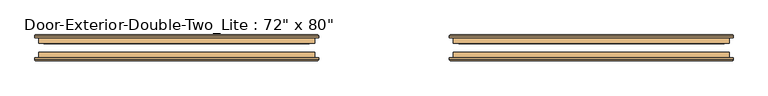
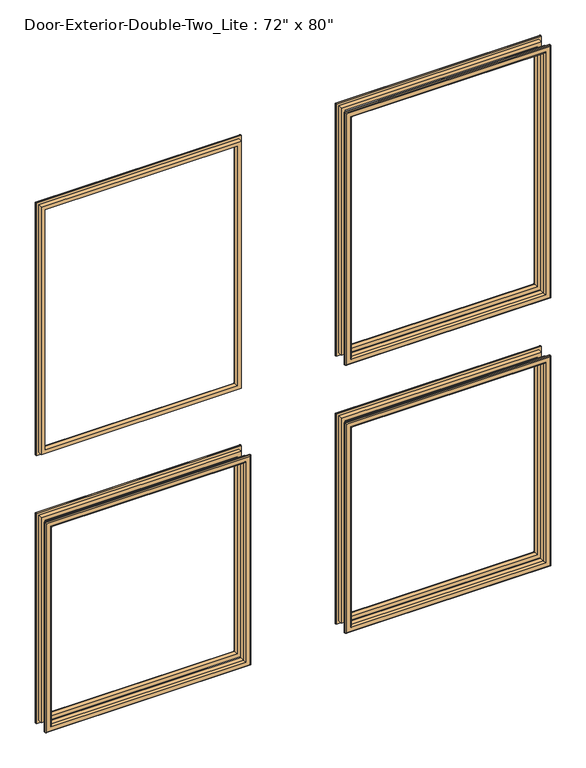
"""IFC4 building model written with IfcOpenShell, lengths in millimetres: door geometry."""

from ifc_helpers import new_model, si_unit, frame, origin, place, context, project, spatial, ellipse_curve, source, transform, mapped, element, save
from ifc_brep_helpers import plane_surface, cylinder_surface, advanced_brep


def door_cb6735bc(model_context):
    return source(origin(), model_context, "Body", "AdvancedBrep", [
        advanced_brep(
        [(-762.0, 69.85, 914.4), (-762.0, 82.55, 914.4), (-762.0, 82.55, 254.0), (-762.0, 69.85, 254.0), (-750.0, 83.55, 902.4), (-750.0, 69.85, 902.4), (-750.0, 69.85, 266.0), (-750.0, 83.55, 266.0), (-755.0, 88.55, 907.4), (-755.0, 88.55, 261.0), (-770.0, 86.55, 922.4), (-768.0, 88.55, 920.4), (-768.0, 88.55, 248.0), (-770.0, 86.55, 246.0), (-770.0, 82.55, 922.4), (-770.0, 82.55, 246.0), (-152.4, 82.55, 254.0), (-152.4, 69.85, 254.0), (-164.4, 69.85, 266.0), (-164.4, 83.55, 266.0), (-159.4, 88.55, 261.0), (-146.4, 88.55, 248.0), (-144.4, 86.55, 246.0), (-144.4, 82.55, 246.0), (-152.4, 82.55, 914.4), (-152.4, 69.85, 914.4), (-164.4, 69.85, 902.4), (-164.4, 83.55, 902.4), (-159.4, 88.55, 907.4), (-146.4, 88.55, 920.4), (-144.4, 86.55, 922.4), (-144.4, 82.55, 922.4)],
        [
            (0, 1),
            (1, 2),
            (2, 3),
            (3, 0),
            (4, 5),
            (5, 6),
            (6, 7),
            (7, 4),
            (8, 4, ellipse_curve(frame((-755.0, 83.55, 907.4), z_axis=(-0.7071067811865475, 0.0, -0.7071067811865475), x_axis=(-0.7071067811865474, 0.0, 0.7071067811865476)), 7.0710678, 5.0)),
            (7, 9, ellipse_curve(frame((-755.0, 83.55, 261.0), z_axis=(-0.7071067811865475, 0.0, 0.7071067811865475), x_axis=(0.7071067811865474, 0.0, 0.7071067811865476)), 7.0710678, 5.0)),
            (9, 8),
            (10, 11, ellipse_curve(frame((-768.0, 86.55, 920.4), z_axis=(-0.7071067811865475, 0.0, -0.7071067811865475), x_axis=(-0.7071067811865474, 0.0, 0.7071067811865476)), 2.8284271, 2.0)),
            (11, 12),
            (12, 13, ellipse_curve(frame((-768.0, 86.55, 248.0), z_axis=(-0.7071067811865475, 0.0, 0.7071067811865475), x_axis=(0.7071067811865474, 0.0, 0.7071067811865476)), 2.8284271, 2.0)),
            (13, 10),
            (14, 10),
            (13, 15),
            (15, 14),
            (2, 16),
            (16, 17),
            (17, 3),
            (6, 18),
            (18, 19),
            (19, 7),
            (19, 20, ellipse_curve(frame((-159.4, 83.55, 261.0), z_axis=(-0.7071067811865475, 0.0, -0.7071067811865475), x_axis=(-0.7071067811865476, 0.0, 0.7071067811865474)), 7.0710678, 5.0)),
            (20, 9),
            (12, 21),
            (21, 22, ellipse_curve(frame((-146.4, 86.55, 248.0), z_axis=(-0.7071067811865475, 0.0, -0.7071067811865475), x_axis=(-0.7071067811865476, 0.0, 0.7071067811865474)), 2.8284271, 2.0)),
            (22, 13),
            (22, 23),
            (23, 15),
            (16, 24),
            (24, 25),
            (25, 17),
            (18, 26),
            (26, 27),
            (27, 19),
            (27, 28, ellipse_curve(frame((-159.4, 83.55, 907.4), z_axis=(0.7071067811865475, 0.0, -0.7071067811865475), x_axis=(-0.7071067811865474, 0.0, -0.7071067811865476)), 7.0710678, 5.0)),
            (28, 20),
            (21, 29),
            (29, 30, ellipse_curve(frame((-146.4, 86.55, 920.4), z_axis=(0.7071067811865475, 0.0, -0.7071067811865475), x_axis=(-0.7071067811865474, 0.0, -0.7071067811865476)), 2.8284271, 2.0)),
            (30, 22),
            (30, 31),
            (31, 23),
            (31, 14),
            (1, 24),
            (0, 25),
            (5, 26),
            (4, 27),
            (8, 28),
            (11, 29),
            (10, 30),
        ],
        [
            plane_surface(frame((-762.0, 82.55, 914.4), z_axis=(-1.0, 0.0, 0.0), x_axis=(0.0, 0.0, -1.0))),
            plane_surface(frame((-750.0, 69.85, 902.4), z_axis=(1.0, 0.0, 0.0), x_axis=(0.0, 0.0, -1.0))),
            cylinder_surface(frame((-755.0, 83.55, 914.4), z_axis=(0.0, 0.0, 1.0), x_axis=(-1.0, 0.0, 0.0)), 5.0),
            cylinder_surface(frame((-768.0, 86.55, 914.4), z_axis=(0.0, 0.0, 1.0), x_axis=(-1.0, 0.0, 0.0)), 2.0),
            plane_surface(frame((-770.0, 86.55, 922.4), z_axis=(-1.0, 0.0, 0.0), x_axis=(0.0, 0.0, -1.0))),
            plane_surface(frame((-762.0, 82.55, 254.0), z_axis=(0.0, 0.0, -1.0), x_axis=(1.0, 0.0, 0.0))),
            plane_surface(frame((-750.0, 69.85, 266.0), z_axis=(0.0, 0.0, 1.0), x_axis=(1.0, 0.0, 0.0))),
            cylinder_surface(frame((-762.0, 83.55, 261.0), z_axis=(-1.0, 0.0, 0.0), x_axis=(0.0, 0.0, -1.0)), 5.0),
            cylinder_surface(frame((-762.0, 86.55, 248.0), z_axis=(-1.0, 0.0, 0.0), x_axis=(0.0, 0.0, -1.0)), 2.0),
            plane_surface(frame((-770.0, 86.55, 246.0), z_axis=(0.0, 0.0, -1.0), x_axis=(1.0, 0.0, 0.0))),
            plane_surface(frame((-152.4, 82.55, 254.0), z_axis=(1.0, 0.0, 0.0), x_axis=(0.0, 0.0, 1.0))),
            plane_surface(frame((-164.4, 69.85, 266.0), z_axis=(-1.0, 0.0, 0.0), x_axis=(0.0, 0.0, 1.0))),
            cylinder_surface(frame((-159.4, 83.55, 254.0), z_axis=(0.0, 0.0, -1.0), x_axis=(1.0, 0.0, 0.0)), 5.0),
            cylinder_surface(frame((-146.4, 86.55, 254.0), z_axis=(0.0, 0.0, -1.0), x_axis=(1.0, 0.0, 0.0)), 2.0),
            plane_surface(frame((-144.4, 86.55, 246.0), z_axis=(1.0, 0.0, 0.0), x_axis=(0.0, 0.0, 1.0))),
            plane_surface(frame((-144.4, 82.55, 922.4), z_axis=(0.0, -1.0, 0.0), x_axis=(-1.0, 0.0, 0.0))),
            plane_surface(frame((-152.4, 82.55, 914.4), z_axis=(0.0, 0.0, 1.0), x_axis=(-1.0, 0.0, 0.0))),
            plane_surface(frame((-152.4, 69.85, 914.4), z_axis=(0.0, -1.0, 0.0), x_axis=(-1.0, 0.0, 0.0))),
            plane_surface(frame((-164.4, 69.85, 902.4), z_axis=(0.0, 0.0, -1.0), x_axis=(-1.0, 0.0, 0.0))),
            cylinder_surface(frame((-152.4, 83.55, 907.4), z_axis=(1.0, 0.0, 0.0), x_axis=(0.0, 0.0, 1.0)), 5.0),
            plane_surface(frame((-159.4, 88.55, 907.4), z_axis=(0.0, 1.0, 0.0), x_axis=(-1.0, 0.0, 0.0))),
            cylinder_surface(frame((-152.4, 86.55, 920.4), z_axis=(1.0, 0.0, 0.0), x_axis=(0.0, 0.0, 1.0)), 2.0),
            plane_surface(frame((-144.4, 86.55, 922.4), z_axis=(0.0, 0.0, 1.0), x_axis=(-1.0, 0.0, 0.0))),
        ],
        [
            (0, [[1, 2, 3, 4]]),
            (1, [[5, 6, 7, 8]]),
            (2, [[9, -8, 10, 11]]),
            (3, [[12, 13, 14, 15]]),
            (4, [[16, -15, 17, 18]]),
            (5, [[-3, 19, 20, 21]]),
            (6, [[-7, 22, 23, 24]]),
            (7, [[-10, -24, 25, 26]]),
            (8, [[-14, 27, 28, 29]]),
            (9, [[-17, -29, 30, 31]]),
            (10, [[-20, 32, 33, 34]]),
            (11, [[-23, 35, 36, 37]]),
            (12, [[-25, -37, 38, 39]]),
            (13, [[-28, 40, 41, 42]]),
            (14, [[-30, -42, 43, 44]]),
            (15, [[-31, -44, 45, -18], [46, -32, -19, -2]]),
            (16, [[-33, -46, -1, 47]]),
            (17, [[-21, -34, -47, -4], [48, -35, -22, -6]]),
            (18, [[-36, -48, -5, 49]]),
            (19, [[-38, -49, -9, 50]]),
            (20, [[51, -40, -27, -13], [-26, -39, -50, -11]]),
            (21, [[-41, -51, -12, 52]]),
            (22, [[-43, -52, -16, -45]]),
        ],
    ),
        advanced_brep(
        [(152.4, 69.85, 914.4), (152.4, 82.55, 914.4), (152.4, 82.55, 254.0), (152.4, 69.85, 254.0), (164.4, 83.55, 902.4), (164.4, 69.85, 902.4), (164.4, 69.85, 266.0), (164.4, 83.55, 266.0), (159.4, 88.55, 907.4), (159.4, 88.55, 261.0), (144.4, 86.55, 922.4), (146.4, 88.55, 920.4), (146.4, 88.55, 248.0), (144.4, 86.55, 246.0), (144.4, 82.55, 922.4), (144.4, 82.55, 246.0), (762.0, 82.55, 254.0), (762.0, 69.85, 254.0), (750.0, 69.85, 266.0), (750.0, 83.55, 266.0), (755.0, 88.55, 261.0), (768.0, 88.55, 248.0), (770.0, 86.55, 246.0), (770.0, 82.55, 246.0), (762.0, 82.55, 914.4), (762.0, 69.85, 914.4), (750.0, 69.85, 902.4), (750.0, 83.55, 902.4), (755.0, 88.55, 907.4), (768.0, 88.55, 920.4), (770.0, 86.55, 922.4), (770.0, 82.55, 922.4)],
        [
            (0, 1),
            (1, 2),
            (2, 3),
            (3, 0),
            (4, 5),
            (5, 6),
            (6, 7),
            (7, 4),
            (8, 4, ellipse_curve(frame((159.4, 83.55, 907.4), z_axis=(-0.7071067811865475, 0.0, -0.7071067811865475), x_axis=(-0.7071067811865474, 0.0, 0.7071067811865476)), 7.0710678, 5.0)),
            (7, 9, ellipse_curve(frame((159.4, 83.55, 261.0), z_axis=(-0.7071067811865475, 0.0, 0.7071067811865475), x_axis=(0.7071067811865474, 0.0, 0.7071067811865476)), 7.0710678, 5.0)),
            (9, 8),
            (10, 11, ellipse_curve(frame((146.4, 86.55, 920.4), z_axis=(-0.7071067811865475, 0.0, -0.7071067811865475), x_axis=(-0.7071067811865474, 0.0, 0.7071067811865476)), 2.8284271, 2.0)),
            (11, 12),
            (12, 13, ellipse_curve(frame((146.4, 86.55, 248.0), z_axis=(-0.7071067811865475, 0.0, 0.7071067811865475), x_axis=(0.7071067811865474, 0.0, 0.7071067811865476)), 2.8284271, 2.0)),
            (13, 10),
            (14, 10),
            (13, 15),
            (15, 14),
            (2, 16),
            (16, 17),
            (17, 3),
            (6, 18),
            (18, 19),
            (19, 7),
            (19, 20, ellipse_curve(frame((755.0, 83.55, 261.0), z_axis=(-0.7071067811865475, 0.0, -0.7071067811865475), x_axis=(-0.7071067811865476, 0.0, 0.7071067811865474)), 7.0710678, 5.0)),
            (20, 9),
            (12, 21),
            (21, 22, ellipse_curve(frame((768.0, 86.55, 248.0), z_axis=(-0.7071067811865475, 0.0, -0.7071067811865475), x_axis=(-0.7071067811865476, 0.0, 0.7071067811865474)), 2.8284271, 2.0)),
            (22, 13),
            (22, 23),
            (23, 15),
            (16, 24),
            (24, 25),
            (25, 17),
            (18, 26),
            (26, 27),
            (27, 19),
            (27, 28, ellipse_curve(frame((755.0, 83.55, 907.4), z_axis=(0.7071067811865475, 0.0, -0.7071067811865475), x_axis=(-0.7071067811865474, 0.0, -0.7071067811865476)), 7.0710678, 5.0)),
            (28, 20),
            (21, 29),
            (29, 30, ellipse_curve(frame((768.0, 86.55, 920.4), z_axis=(0.7071067811865475, 0.0, -0.7071067811865475), x_axis=(-0.7071067811865474, 0.0, -0.7071067811865476)), 2.8284271, 2.0)),
            (30, 22),
            (30, 31),
            (31, 23),
            (31, 14),
            (1, 24),
            (0, 25),
            (5, 26),
            (4, 27),
            (8, 28),
            (11, 29),
            (10, 30),
        ],
        [
            plane_surface(frame((152.4, 82.55, 914.4), z_axis=(-1.0, 0.0, 0.0), x_axis=(0.0, 0.0, -1.0))),
            plane_surface(frame((164.4, 69.85, 902.4), z_axis=(1.0, 0.0, 0.0), x_axis=(0.0, 0.0, -1.0))),
            cylinder_surface(frame((159.4, 83.55, 914.4), z_axis=(0.0, 0.0, 1.0), x_axis=(-1.0, 0.0, 0.0)), 5.0),
            cylinder_surface(frame((146.4, 86.55, 914.4), z_axis=(0.0, 0.0, 1.0), x_axis=(-1.0, 0.0, 0.0)), 2.0),
            plane_surface(frame((144.4, 86.55, 922.4), z_axis=(-1.0, 0.0, 0.0), x_axis=(0.0, 0.0, -1.0))),
            plane_surface(frame((152.4, 82.55, 254.0), z_axis=(0.0, 0.0, -1.0), x_axis=(1.0, 0.0, 0.0))),
            plane_surface(frame((164.4, 69.85, 266.0), z_axis=(0.0, 0.0, 1.0), x_axis=(1.0, 0.0, 0.0))),
            cylinder_surface(frame((152.4, 83.55, 261.0), z_axis=(-1.0, 0.0, 0.0), x_axis=(0.0, 0.0, -1.0)), 5.0),
            cylinder_surface(frame((152.4, 86.55, 248.0), z_axis=(-1.0, 0.0, 0.0), x_axis=(0.0, 0.0, -1.0)), 2.0),
            plane_surface(frame((144.4, 86.55, 246.0), z_axis=(0.0, 0.0, -1.0), x_axis=(1.0, 0.0, 0.0))),
            plane_surface(frame((762.0, 82.55, 254.0), z_axis=(1.0, 0.0, 0.0), x_axis=(0.0, 0.0, 1.0))),
            plane_surface(frame((750.0, 69.85, 266.0), z_axis=(-1.0, 0.0, 0.0), x_axis=(0.0, 0.0, 1.0))),
            cylinder_surface(frame((755.0, 83.55, 254.0), z_axis=(0.0, 0.0, -1.0), x_axis=(1.0, 0.0, 0.0)), 5.0),
            cylinder_surface(frame((768.0, 86.55, 254.0), z_axis=(0.0, 0.0, -1.0), x_axis=(1.0, 0.0, 0.0)), 2.0),
            plane_surface(frame((770.0, 86.55, 246.0), z_axis=(1.0, 0.0, 0.0), x_axis=(0.0, 0.0, 1.0))),
            plane_surface(frame((770.0, 82.55, 922.4), z_axis=(0.0, -1.0, 0.0), x_axis=(-1.0, 0.0, 0.0))),
            plane_surface(frame((762.0, 82.55, 914.4), z_axis=(0.0, 0.0, 1.0), x_axis=(-1.0, 0.0, 0.0))),
            plane_surface(frame((762.0, 69.85, 914.4), z_axis=(0.0, -1.0, 0.0), x_axis=(-1.0, 0.0, 0.0))),
            plane_surface(frame((750.0, 69.85, 902.4), z_axis=(0.0, 0.0, -1.0), x_axis=(-1.0, 0.0, 0.0))),
            cylinder_surface(frame((762.0, 83.55, 907.4), z_axis=(1.0, 0.0, 0.0), x_axis=(0.0, 0.0, 1.0)), 5.0),
            plane_surface(frame((755.0, 88.55, 907.4), z_axis=(0.0, 1.0, 0.0), x_axis=(-1.0, 0.0, 0.0))),
            cylinder_surface(frame((762.0, 86.55, 920.4), z_axis=(1.0, 0.0, 0.0), x_axis=(0.0, 0.0, 1.0)), 2.0),
            plane_surface(frame((770.0, 86.55, 922.4), z_axis=(0.0, 0.0, 1.0), x_axis=(-1.0, 0.0, 0.0))),
        ],
        [
            (0, [[1, 2, 3, 4]]),
            (1, [[5, 6, 7, 8]]),
            (2, [[9, -8, 10, 11]]),
            (3, [[12, 13, 14, 15]]),
            (4, [[16, -15, 17, 18]]),
            (5, [[-3, 19, 20, 21]]),
            (6, [[-7, 22, 23, 24]]),
            (7, [[-10, -24, 25, 26]]),
            (8, [[-14, 27, 28, 29]]),
            (9, [[-17, -29, 30, 31]]),
            (10, [[-20, 32, 33, 34]]),
            (11, [[-23, 35, 36, 37]]),
            (12, [[-25, -37, 38, 39]]),
            (13, [[-28, 40, 41, 42]]),
            (14, [[-30, -42, 43, 44]]),
            (15, [[-31, -44, 45, -18], [46, -32, -19, -2]]),
            (16, [[-33, -46, -1, 47]]),
            (17, [[-21, -34, -47, -4], [48, -35, -22, -6]]),
            (18, [[-36, -48, -5, 49]]),
            (19, [[-38, -49, -9, 50]]),
            (20, [[51, -40, -27, -13], [-26, -39, -50, -11]]),
            (21, [[-41, -51, -12, 52]]),
            (22, [[-43, -52, -16, -45]]),
        ],
    ),
        advanced_brep(
        [(152.4, 69.85, 1914.525), (152.4, 82.55, 1914.525), (152.4, 82.55, 1117.6), (152.4, 69.85, 1117.6), (164.4, 83.55, 1902.525), (164.4, 69.85, 1902.525), (164.4, 69.85, 1129.6), (164.4, 83.55, 1129.6), (159.4, 88.55, 1907.525), (159.4, 88.55, 1124.6), (144.4, 86.55, 1922.525), (146.4, 88.55, 1920.525), (146.4, 88.55, 1111.6), (144.4, 86.55, 1109.6), (144.4, 82.55, 1922.525), (144.4, 82.55, 1109.6), (762.0, 82.55, 1117.6), (762.0, 69.85, 1117.6), (750.0, 69.85, 1129.6), (750.0, 83.55, 1129.6), (755.0, 88.55, 1124.6), (768.0, 88.55, 1111.6), (770.0, 86.55, 1109.6), (770.0, 82.55, 1109.6), (762.0, 82.55, 1914.525), (762.0, 69.85, 1914.525), (750.0, 69.85, 1902.525), (750.0, 83.55, 1902.525), (755.0, 88.55, 1907.525), (768.0, 88.55, 1920.525), (770.0, 86.55, 1922.525), (770.0, 82.55, 1922.525)],
        [
            (0, 1),
            (1, 2),
            (2, 3),
            (3, 0),
            (4, 5),
            (5, 6),
            (6, 7),
            (7, 4),
            (8, 4, ellipse_curve(frame((159.4, 83.55, 1907.525), z_axis=(-0.7071067811865475, 0.0, -0.7071067811865475), x_axis=(-0.7071067811865474, 0.0, 0.7071067811865476)), 7.0710678, 5.0)),
            (7, 9, ellipse_curve(frame((159.4, 83.55, 1124.6), z_axis=(-0.7071067811865475, 0.0, 0.7071067811865475), x_axis=(0.7071067811865474, 0.0, 0.7071067811865476)), 7.0710678, 5.0)),
            (9, 8),
            (10, 11, ellipse_curve(frame((146.4, 86.55, 1920.525), z_axis=(-0.7071067811865475, 0.0, -0.7071067811865475), x_axis=(-0.7071067811865474, 0.0, 0.7071067811865476)), 2.8284271, 2.0)),
            (11, 12),
            (12, 13, ellipse_curve(frame((146.4, 86.55, 1111.6), z_axis=(-0.7071067811865475, 0.0, 0.7071067811865475), x_axis=(0.7071067811865474, 0.0, 0.7071067811865476)), 2.8284271, 2.0)),
            (13, 10),
            (14, 10),
            (13, 15),
            (15, 14),
            (2, 16),
            (16, 17),
            (17, 3),
            (6, 18),
            (18, 19),
            (19, 7),
            (19, 20, ellipse_curve(frame((755.0, 83.55, 1124.6), z_axis=(-0.7071067811865475, 0.0, -0.7071067811865475), x_axis=(-0.7071067811865476, 0.0, 0.7071067811865474)), 7.0710678, 5.0)),
            (20, 9),
            (12, 21),
            (21, 22, ellipse_curve(frame((768.0, 86.55, 1111.6), z_axis=(-0.7071067811865475, 0.0, -0.7071067811865475), x_axis=(-0.7071067811865476, 0.0, 0.7071067811865474)), 2.8284271, 2.0)),
            (22, 13),
            (22, 23),
            (23, 15),
            (16, 24),
            (24, 25),
            (25, 17),
            (18, 26),
            (26, 27),
            (27, 19),
            (27, 28, ellipse_curve(frame((755.0, 83.55, 1907.525), z_axis=(0.7071067811865475, 0.0, -0.7071067811865475), x_axis=(-0.7071067811865474, 0.0, -0.7071067811865476)), 7.0710678, 5.0)),
            (28, 20),
            (21, 29),
            (29, 30, ellipse_curve(frame((768.0, 86.55, 1920.525), z_axis=(0.7071067811865475, 0.0, -0.7071067811865475), x_axis=(-0.7071067811865474, 0.0, -0.7071067811865476)), 2.8284271, 2.0)),
            (30, 22),
            (30, 31),
            (31, 23),
            (31, 14),
            (1, 24),
            (0, 25),
            (5, 26),
            (4, 27),
            (8, 28),
            (11, 29),
            (10, 30),
        ],
        [
            plane_surface(frame((152.4, 82.55, 1914.525), z_axis=(-1.0, 0.0, 0.0), x_axis=(0.0, 0.0, -1.0))),
            plane_surface(frame((164.4, 69.85, 1902.525), z_axis=(1.0, 0.0, 0.0), x_axis=(0.0, 0.0, -1.0))),
            cylinder_surface(frame((159.4, 83.55, 1914.525), z_axis=(0.0, 0.0, 1.0), x_axis=(-1.0, 0.0, 0.0)), 5.0),
            cylinder_surface(frame((146.4, 86.55, 1914.525), z_axis=(0.0, 0.0, 1.0), x_axis=(-1.0, 0.0, 0.0)), 2.0),
            plane_surface(frame((144.4, 86.55, 1922.525), z_axis=(-1.0, 0.0, 0.0), x_axis=(0.0, 0.0, -1.0))),
            plane_surface(frame((152.4, 82.55, 1117.6), z_axis=(0.0, 0.0, -1.0), x_axis=(1.0, 0.0, 0.0))),
            plane_surface(frame((164.4, 69.85, 1129.6), z_axis=(0.0, 0.0, 1.0), x_axis=(1.0, 0.0, 0.0))),
            cylinder_surface(frame((152.4, 83.55, 1124.6), z_axis=(-1.0, 0.0, 0.0), x_axis=(0.0, 0.0, -1.0)), 5.0),
            cylinder_surface(frame((152.4, 86.55, 1111.6), z_axis=(-1.0, 0.0, 0.0), x_axis=(0.0, 0.0, -1.0)), 2.0),
            plane_surface(frame((144.4, 86.55, 1109.6), z_axis=(0.0, 0.0, -1.0), x_axis=(1.0, 0.0, 0.0))),
            plane_surface(frame((762.0, 82.55, 1117.6), z_axis=(1.0, 0.0, 0.0), x_axis=(0.0, 0.0, 1.0))),
            plane_surface(frame((750.0, 69.85, 1129.6), z_axis=(-1.0, 0.0, 0.0), x_axis=(0.0, 0.0, 1.0))),
            cylinder_surface(frame((755.0, 83.55, 1117.6), z_axis=(0.0, 0.0, -1.0), x_axis=(1.0, 0.0, 0.0)), 5.0),
            cylinder_surface(frame((768.0, 86.55, 1117.6), z_axis=(0.0, 0.0, -1.0), x_axis=(1.0, 0.0, 0.0)), 2.0),
            plane_surface(frame((770.0, 86.55, 1109.6), z_axis=(1.0, 0.0, 0.0), x_axis=(0.0, 0.0, 1.0))),
            plane_surface(frame((770.0, 82.55, 1922.525), z_axis=(0.0, -1.0, 0.0), x_axis=(-1.0, 0.0, 0.0))),
            plane_surface(frame((762.0, 82.55, 1914.525), z_axis=(0.0, 0.0, 1.0), x_axis=(-1.0, 0.0, 0.0))),
            plane_surface(frame((762.0, 69.85, 1914.525), z_axis=(0.0, -1.0, 0.0), x_axis=(-1.0, 0.0, 0.0))),
            plane_surface(frame((750.0, 69.85, 1902.525), z_axis=(0.0, 0.0, -1.0), x_axis=(-1.0, 0.0, 0.0))),
            cylinder_surface(frame((762.0, 83.55, 1907.525), z_axis=(1.0, 0.0, 0.0), x_axis=(0.0, 0.0, 1.0)), 5.0),
            plane_surface(frame((755.0, 88.55, 1907.525), z_axis=(0.0, 1.0, 0.0), x_axis=(-1.0, 0.0, 0.0))),
            cylinder_surface(frame((762.0, 86.55, 1920.525), z_axis=(1.0, 0.0, 0.0), x_axis=(0.0, 0.0, 1.0)), 2.0),
            plane_surface(frame((770.0, 86.55, 1922.525), z_axis=(0.0, 0.0, 1.0), x_axis=(-1.0, 0.0, 0.0))),
        ],
        [
            (0, [[1, 2, 3, 4]]),
            (1, [[5, 6, 7, 8]]),
            (2, [[9, -8, 10, 11]]),
            (3, [[12, 13, 14, 15]]),
            (4, [[16, -15, 17, 18]]),
            (5, [[-3, 19, 20, 21]]),
            (6, [[-7, 22, 23, 24]]),
            (7, [[-10, -24, 25, 26]]),
            (8, [[-14, 27, 28, 29]]),
            (9, [[-17, -29, 30, 31]]),
            (10, [[-20, 32, 33, 34]]),
            (11, [[-23, 35, 36, 37]]),
            (12, [[-25, -37, 38, 39]]),
            (13, [[-28, 40, 41, 42]]),
            (14, [[-30, -42, 43, 44]]),
            (15, [[-31, -44, 45, -18], [46, -32, -19, -2]]),
            (16, [[-33, -46, -1, 47]]),
            (17, [[-21, -34, -47, -4], [48, -35, -22, -6]]),
            (18, [[-36, -48, -5, 49]]),
            (19, [[-38, -49, -9, 50]]),
            (20, [[51, -40, -27, -13], [-26, -39, -50, -11]]),
            (21, [[-41, -51, -12, 52]]),
            (22, [[-43, -52, -16, -45]]),
        ],
    ),
        advanced_brep(
        [(-762.0, 69.85, 1914.525), (-762.0, 82.55, 1914.525), (-762.0, 82.55, 1117.6), (-762.0, 69.85, 1117.6), (-750.0, 83.55, 1902.525), (-750.0, 69.85, 1902.525), (-750.0, 69.85, 1129.6), (-750.0, 83.55, 1129.6), (-755.0, 88.55, 1907.525), (-755.0, 88.55, 1124.6), (-770.0, 86.55, 1922.525), (-768.0, 88.55, 1920.525), (-768.0, 88.55, 1111.6), (-770.0, 86.55, 1109.6), (-770.0, 82.55, 1922.525), (-770.0, 82.55, 1109.6), (-152.4, 82.55, 1117.6), (-152.4, 69.85, 1117.6), (-164.4, 69.85, 1129.6), (-164.4, 83.55, 1129.6), (-159.4, 88.55, 1124.6), (-146.4, 88.55, 1111.6), (-144.4, 86.55, 1109.6), (-144.4, 82.55, 1109.6), (-152.4, 82.55, 1914.525), (-152.4, 69.85, 1914.525), (-164.4, 69.85, 1902.525), (-164.4, 83.55, 1902.525), (-159.4, 88.55, 1907.525), (-146.4, 88.55, 1920.525), (-144.4, 86.55, 1922.525), (-144.4, 82.55, 1922.525)],
        [
            (0, 1),
            (1, 2),
            (2, 3),
            (3, 0),
            (4, 5),
            (5, 6),
            (6, 7),
            (7, 4),
            (8, 4, ellipse_curve(frame((-755.0, 83.55, 1907.525), z_axis=(-0.7071067811865475, 0.0, -0.7071067811865475), x_axis=(-0.7071067811865474, 0.0, 0.7071067811865476)), 7.0710678, 5.0)),
            (7, 9, ellipse_curve(frame((-755.0, 83.55, 1124.6), z_axis=(-0.7071067811865475, 0.0, 0.7071067811865475), x_axis=(0.7071067811865474, 0.0, 0.7071067811865476)), 7.0710678, 5.0)),
            (9, 8),
            (10, 11, ellipse_curve(frame((-768.0, 86.55, 1920.525), z_axis=(-0.7071067811865475, 0.0, -0.7071067811865475), x_axis=(-0.7071067811865474, 0.0, 0.7071067811865476)), 2.8284271, 2.0)),
            (11, 12),
            (12, 13, ellipse_curve(frame((-768.0, 86.55, 1111.6), z_axis=(-0.7071067811865475, 0.0, 0.7071067811865475), x_axis=(0.7071067811865474, 0.0, 0.7071067811865476)), 2.8284271, 2.0)),
            (13, 10),
            (14, 10),
            (13, 15),
            (15, 14),
            (2, 16),
            (16, 17),
            (17, 3),
            (6, 18),
            (18, 19),
            (19, 7),
            (19, 20, ellipse_curve(frame((-159.4, 83.55, 1124.6), z_axis=(-0.7071067811865475, 0.0, -0.7071067811865475), x_axis=(-0.7071067811865476, 0.0, 0.7071067811865474)), 7.0710678, 5.0)),
            (20, 9),
            (12, 21),
            (21, 22, ellipse_curve(frame((-146.4, 86.55, 1111.6), z_axis=(-0.7071067811865475, 0.0, -0.7071067811865475), x_axis=(-0.7071067811865476, 0.0, 0.7071067811865474)), 2.8284271, 2.0)),
            (22, 13),
            (22, 23),
            (23, 15),
            (16, 24),
            (24, 25),
            (25, 17),
            (18, 26),
            (26, 27),
            (27, 19),
            (27, 28, ellipse_curve(frame((-159.4, 83.55, 1907.525), z_axis=(0.7071067811865475, 0.0, -0.7071067811865475), x_axis=(-0.7071067811865474, 0.0, -0.7071067811865476)), 7.0710678, 5.0)),
            (28, 20),
            (21, 29),
            (29, 30, ellipse_curve(frame((-146.4, 86.55, 1920.525), z_axis=(0.7071067811865475, 0.0, -0.7071067811865475), x_axis=(-0.7071067811865474, 0.0, -0.7071067811865476)), 2.8284271, 2.0)),
            (30, 22),
            (30, 31),
            (31, 23),
            (31, 14),
            (1, 24),
            (0, 25),
            (5, 26),
            (4, 27),
            (8, 28),
            (11, 29),
            (10, 30),
        ],
        [
            plane_surface(frame((-762.0, 82.55, 1914.525), z_axis=(-1.0, 0.0, 0.0), x_axis=(0.0, 0.0, -1.0))),
            plane_surface(frame((-750.0, 69.85, 1902.525), z_axis=(1.0, 0.0, 0.0), x_axis=(0.0, 0.0, -1.0))),
            cylinder_surface(frame((-755.0, 83.55, 1914.525), z_axis=(0.0, 0.0, 1.0), x_axis=(-1.0, 0.0, 0.0)), 5.0),
            cylinder_surface(frame((-768.0, 86.55, 1914.525), z_axis=(0.0, 0.0, 1.0), x_axis=(-1.0, 0.0, 0.0)), 2.0),
            plane_surface(frame((-770.0, 86.55, 1922.525), z_axis=(-1.0, 0.0, 0.0), x_axis=(0.0, 0.0, -1.0))),
            plane_surface(frame((-762.0, 82.55, 1117.6), z_axis=(0.0, 0.0, -1.0), x_axis=(1.0, 0.0, 0.0))),
            plane_surface(frame((-750.0, 69.85, 1129.6), z_axis=(0.0, 0.0, 1.0), x_axis=(1.0, 0.0, 0.0))),
            cylinder_surface(frame((-762.0, 83.55, 1124.6), z_axis=(-1.0, 0.0, 0.0), x_axis=(0.0, 0.0, -1.0)), 5.0),
            cylinder_surface(frame((-762.0, 86.55, 1111.6), z_axis=(-1.0, 0.0, 0.0), x_axis=(0.0, 0.0, -1.0)), 2.0),
            plane_surface(frame((-770.0, 86.55, 1109.6), z_axis=(0.0, 0.0, -1.0), x_axis=(1.0, 0.0, 0.0))),
            plane_surface(frame((-152.4, 82.55, 1117.6), z_axis=(1.0, 0.0, 0.0), x_axis=(0.0, 0.0, 1.0))),
            plane_surface(frame((-164.4, 69.85, 1129.6), z_axis=(-1.0, 0.0, 0.0), x_axis=(0.0, 0.0, 1.0))),
            cylinder_surface(frame((-159.4, 83.55, 1117.6), z_axis=(0.0, 0.0, -1.0), x_axis=(1.0, 0.0, 0.0)), 5.0),
            cylinder_surface(frame((-146.4, 86.55, 1117.6), z_axis=(0.0, 0.0, -1.0), x_axis=(1.0, 0.0, 0.0)), 2.0),
            plane_surface(frame((-144.4, 86.55, 1109.6), z_axis=(1.0, 0.0, 0.0), x_axis=(0.0, 0.0, 1.0))),
            plane_surface(frame((-144.4, 82.55, 1922.525), z_axis=(0.0, -1.0, 0.0), x_axis=(-1.0, 0.0, 0.0))),
            plane_surface(frame((-152.4, 82.55, 1914.525), z_axis=(0.0, 0.0, 1.0), x_axis=(-1.0, 0.0, 0.0))),
            plane_surface(frame((-152.4, 69.85, 1914.525), z_axis=(0.0, -1.0, 0.0), x_axis=(-1.0, 0.0, 0.0))),
            plane_surface(frame((-164.4, 69.85, 1902.525), z_axis=(0.0, 0.0, -1.0), x_axis=(-1.0, 0.0, 0.0))),
            cylinder_surface(frame((-152.4, 83.55, 1907.525), z_axis=(1.0, 0.0, 0.0), x_axis=(0.0, 0.0, 1.0)), 5.0),
            plane_surface(frame((-159.4, 88.55, 1907.525), z_axis=(0.0, 1.0, 0.0), x_axis=(-1.0, 0.0, 0.0))),
            cylinder_surface(frame((-152.4, 86.55, 1920.525), z_axis=(1.0, 0.0, 0.0), x_axis=(0.0, 0.0, 1.0)), 2.0),
            plane_surface(frame((-144.4, 86.55, 1922.525), z_axis=(0.0, 0.0, 1.0), x_axis=(-1.0, 0.0, 0.0))),
        ],
        [
            (0, [[1, 2, 3, 4]]),
            (1, [[5, 6, 7, 8]]),
            (2, [[9, -8, 10, 11]]),
            (3, [[12, 13, 14, 15]]),
            (4, [[16, -15, 17, 18]]),
            (5, [[-3, 19, 20, 21]]),
            (6, [[-7, 22, 23, 24]]),
            (7, [[-10, -24, 25, 26]]),
            (8, [[-14, 27, 28, 29]]),
            (9, [[-17, -29, 30, 31]]),
            (10, [[-20, 32, 33, 34]]),
            (11, [[-23, 35, 36, 37]]),
            (12, [[-25, -37, 38, 39]]),
            (13, [[-28, 40, 41, 42]]),
            (14, [[-30, -42, 43, 44]]),
            (15, [[-31, -44, 45, -18], [46, -32, -19, -2]]),
            (16, [[-33, -46, -1, 47]]),
            (17, [[-21, -34, -47, -4], [48, -35, -22, -6]]),
            (18, [[-36, -48, -5, 49]]),
            (19, [[-38, -49, -9, 50]]),
            (20, [[51, -40, -27, -13], [-26, -39, -50, -11]]),
            (21, [[-41, -51, -12, 52]]),
            (22, [[-43, -52, -16, -45]]),
        ],
    ),
        advanced_brep(
        [(-762.0, 50.8, 254.0), (-762.0, 38.1, 254.0), (-762.0, 38.1, 914.4), (-762.0, 50.8, 914.4), (-750.0, 37.1, 266.0), (-750.0, 50.8, 266.0), (-750.0, 50.8, 902.4), (-750.0, 37.1, 902.4), (-755.0, 32.1, 261.0), (-755.0, 32.1, 907.4), (-770.0, 34.1, 246.0), (-768.0, 32.1, 248.0), (-768.0, 32.1, 920.4), (-770.0, 34.1, 922.4), (-770.0, 38.1, 246.0), (-770.0, 38.1, 922.4), (-152.4, 38.1, 914.4), (-152.4, 50.8, 914.4), (-164.4, 50.8, 902.4), (-164.4, 37.1, 902.4), (-159.4, 32.1, 907.4), (-146.4, 32.1, 920.4), (-144.4, 34.1, 922.4), (-144.4, 38.1, 922.4), (-152.4, 38.1, 254.0), (-152.4, 50.8, 254.0), (-164.4, 50.8, 266.0), (-164.4, 37.1, 266.0), (-159.4, 32.1, 261.0), (-146.4, 32.1, 248.0), (-144.4, 34.1, 246.0), (-144.4, 38.1, 246.0)],
        [
            (0, 1),
            (1, 2),
            (2, 3),
            (3, 0),
            (4, 5),
            (5, 6),
            (6, 7),
            (7, 4),
            (8, 4, ellipse_curve(frame((-755.0, 37.1, 261.0), z_axis=(-0.7071067811865475, 0.0, 0.7071067811865475), x_axis=(-0.7071067811865474, 0.0, -0.7071067811865476)), 7.0710678, 5.0)),
            (7, 9, ellipse_curve(frame((-755.0, 37.1, 907.4), z_axis=(-0.7071067811865475, 0.0, -0.7071067811865475), x_axis=(0.7071067811865474, 0.0, -0.7071067811865476)), 7.0710678, 5.0)),
            (9, 8),
            (10, 11, ellipse_curve(frame((-768.0, 34.1, 248.0), z_axis=(-0.7071067811865475, 0.0, 0.7071067811865475), x_axis=(-0.7071067811865474, 0.0, -0.7071067811865476)), 2.8284271, 2.0)),
            (11, 12),
            (12, 13, ellipse_curve(frame((-768.0, 34.1, 920.4), z_axis=(-0.7071067811865475, 0.0, -0.7071067811865475), x_axis=(0.7071067811865474, 0.0, -0.7071067811865476)), 2.8284271, 2.0)),
            (13, 10),
            (14, 10),
            (13, 15),
            (15, 14),
            (2, 16),
            (16, 17),
            (17, 3),
            (6, 18),
            (18, 19),
            (19, 7),
            (19, 20, ellipse_curve(frame((-159.4, 37.1, 907.4), z_axis=(-0.7071067811865475, 0.0, 0.7071067811865475), x_axis=(-0.7071067811865476, 0.0, -0.7071067811865474)), 7.0710678, 5.0)),
            (20, 9),
            (12, 21),
            (21, 22, ellipse_curve(frame((-146.4, 34.1, 920.4), z_axis=(-0.7071067811865475, 0.0, 0.7071067811865475), x_axis=(-0.7071067811865476, 0.0, -0.7071067811865474)), 2.8284271, 2.0)),
            (22, 13),
            (22, 23),
            (23, 15),
            (16, 24),
            (24, 25),
            (25, 17),
            (18, 26),
            (26, 27),
            (27, 19),
            (27, 28, ellipse_curve(frame((-159.4, 37.1, 261.0), z_axis=(0.7071067811865475, 0.0, 0.7071067811865475), x_axis=(-0.7071067811865474, 0.0, 0.7071067811865476)), 7.0710678, 5.0)),
            (28, 20),
            (21, 29),
            (29, 30, ellipse_curve(frame((-146.4, 34.1, 248.0), z_axis=(0.7071067811865475, 0.0, 0.7071067811865475), x_axis=(-0.7071067811865474, 0.0, 0.7071067811865476)), 2.8284271, 2.0)),
            (30, 22),
            (30, 31),
            (31, 23),
            (31, 14),
            (1, 24),
            (0, 25),
            (5, 26),
            (4, 27),
            (8, 28),
            (11, 29),
            (10, 30),
        ],
        [
            plane_surface(frame((-762.0, 38.1, 254.0), z_axis=(-1.0, 0.0, 0.0), x_axis=(0.0, 0.0, 1.0))),
            plane_surface(frame((-750.0, 50.8, 266.0), z_axis=(1.0, 0.0, 0.0), x_axis=(0.0, 0.0, 1.0))),
            cylinder_surface(frame((-755.0, 37.1, 254.0), z_axis=(0.0, 0.0, -1.0), x_axis=(-1.0, 0.0, 0.0)), 5.0),
            cylinder_surface(frame((-768.0, 34.1, 254.0), z_axis=(0.0, 0.0, -1.0), x_axis=(-1.0, 0.0, 0.0)), 2.0),
            plane_surface(frame((-770.0, 34.1, 246.0), z_axis=(-1.0, 0.0, 0.0), x_axis=(0.0, 0.0, 1.0))),
            plane_surface(frame((-762.0, 38.1, 914.4), z_axis=(0.0, 0.0, 1.0), x_axis=(1.0, 0.0, 0.0))),
            plane_surface(frame((-750.0, 50.8, 902.4), z_axis=(0.0, 0.0, -1.0), x_axis=(1.0, 0.0, 0.0))),
            cylinder_surface(frame((-762.0, 37.1, 907.4), z_axis=(-1.0, 0.0, 0.0), x_axis=(0.0, 0.0, 1.0)), 5.0),
            cylinder_surface(frame((-762.0, 34.1, 920.4), z_axis=(-1.0, 0.0, 0.0), x_axis=(0.0, 0.0, 1.0)), 2.0),
            plane_surface(frame((-770.0, 34.1, 922.4), z_axis=(0.0, 0.0, 1.0), x_axis=(1.0, 0.0, 0.0))),
            plane_surface(frame((-152.4, 38.1, 914.4), z_axis=(1.0, 0.0, 0.0), x_axis=(0.0, 0.0, -1.0))),
            plane_surface(frame((-164.4, 50.8, 902.4), z_axis=(-1.0, 0.0, 0.0), x_axis=(0.0, 0.0, -1.0))),
            cylinder_surface(frame((-159.4, 37.1, 914.4), z_axis=(0.0, 0.0, 1.0), x_axis=(1.0, 0.0, 0.0)), 5.0),
            cylinder_surface(frame((-146.4, 34.1, 914.4), z_axis=(0.0, 0.0, 1.0), x_axis=(1.0, 0.0, 0.0)), 2.0),
            plane_surface(frame((-144.4, 34.1, 922.4), z_axis=(1.0, 0.0, 0.0), x_axis=(0.0, 0.0, -1.0))),
            plane_surface(frame((-144.4, 38.1, 246.0), z_axis=(0.0, 1.0, 0.0), x_axis=(-1.0, 0.0, 0.0))),
            plane_surface(frame((-152.4, 38.1, 254.0), z_axis=(0.0, 0.0, -1.0), x_axis=(-1.0, 0.0, 0.0))),
            plane_surface(frame((-152.4, 50.8, 254.0), z_axis=(0.0, 1.0, 0.0), x_axis=(-1.0, 0.0, 0.0))),
            plane_surface(frame((-164.4, 50.8, 266.0), z_axis=(0.0, 0.0, 1.0), x_axis=(-1.0, 0.0, 0.0))),
            cylinder_surface(frame((-152.4, 37.1, 261.0), z_axis=(1.0, 0.0, 0.0), x_axis=(0.0, 0.0, -1.0)), 5.0),
            plane_surface(frame((-159.4, 32.1, 261.0), z_axis=(0.0, -1.0, 0.0), x_axis=(-1.0, 0.0, 0.0))),
            cylinder_surface(frame((-152.4, 34.1, 248.0), z_axis=(1.0, 0.0, 0.0), x_axis=(0.0, 0.0, -1.0)), 2.0),
            plane_surface(frame((-144.4, 34.1, 246.0), z_axis=(0.0, 0.0, -1.0), x_axis=(-1.0, 0.0, 0.0))),
        ],
        [
            (0, [[1, 2, 3, 4]]),
            (1, [[5, 6, 7, 8]]),
            (2, [[9, -8, 10, 11]]),
            (3, [[12, 13, 14, 15]]),
            (4, [[16, -15, 17, 18]]),
            (5, [[-3, 19, 20, 21]]),
            (6, [[-7, 22, 23, 24]]),
            (7, [[-10, -24, 25, 26]]),
            (8, [[-14, 27, 28, 29]]),
            (9, [[-17, -29, 30, 31]]),
            (10, [[-20, 32, 33, 34]]),
            (11, [[-23, 35, 36, 37]]),
            (12, [[-25, -37, 38, 39]]),
            (13, [[-28, 40, 41, 42]]),
            (14, [[-30, -42, 43, 44]]),
            (15, [[-31, -44, 45, -18], [46, -32, -19, -2]]),
            (16, [[-33, -46, -1, 47]]),
            (17, [[-21, -34, -47, -4], [48, -35, -22, -6]]),
            (18, [[-36, -48, -5, 49]]),
            (19, [[-38, -49, -9, 50]]),
            (20, [[51, -40, -27, -13], [-26, -39, -50, -11]]),
            (21, [[-41, -51, -12, 52]]),
            (22, [[-43, -52, -16, -45]]),
        ],
    ),
        advanced_brep(
        [(152.4, 50.8, 254.0), (152.4, 38.1, 254.0), (152.4, 38.1, 914.4), (152.4, 50.8, 914.4), (164.4, 37.1, 266.0), (164.4, 50.8, 266.0), (164.4, 50.8, 902.4), (164.4, 37.1, 902.4), (159.4, 32.1, 261.0), (159.4, 32.1, 907.4), (144.4, 34.1, 246.0), (146.4, 32.1, 248.0), (146.4, 32.1, 920.4), (144.4, 34.1, 922.4), (144.4, 38.1, 246.0), (144.4, 38.1, 922.4), (762.0, 38.1, 914.4), (762.0, 50.8, 914.4), (750.0, 50.8, 902.4), (750.0, 37.1, 902.4), (755.0, 32.1, 907.4), (768.0, 32.1, 920.4), (770.0, 34.1, 922.4), (770.0, 38.1, 922.4), (762.0, 38.1, 254.0), (762.0, 50.8, 254.0), (750.0, 50.8, 266.0), (750.0, 37.1, 266.0), (755.0, 32.1, 261.0), (768.0, 32.1, 248.0), (770.0, 34.1, 246.0), (770.0, 38.1, 246.0)],
        [
            (0, 1),
            (1, 2),
            (2, 3),
            (3, 0),
            (4, 5),
            (5, 6),
            (6, 7),
            (7, 4),
            (8, 4, ellipse_curve(frame((159.4, 37.1, 261.0), z_axis=(-0.7071067811865475, 0.0, 0.7071067811865475), x_axis=(-0.7071067811865474, 0.0, -0.7071067811865476)), 7.0710678, 5.0)),
            (7, 9, ellipse_curve(frame((159.4, 37.1, 907.4), z_axis=(-0.7071067811865475, 0.0, -0.7071067811865475), x_axis=(0.7071067811865474, 0.0, -0.7071067811865476)), 7.0710678, 5.0)),
            (9, 8),
            (10, 11, ellipse_curve(frame((146.4, 34.1, 248.0), z_axis=(-0.7071067811865475, 0.0, 0.7071067811865475), x_axis=(-0.7071067811865474, 0.0, -0.7071067811865476)), 2.8284271, 2.0)),
            (11, 12),
            (12, 13, ellipse_curve(frame((146.4, 34.1, 920.4), z_axis=(-0.7071067811865475, 0.0, -0.7071067811865475), x_axis=(0.7071067811865474, 0.0, -0.7071067811865476)), 2.8284271, 2.0)),
            (13, 10),
            (14, 10),
            (13, 15),
            (15, 14),
            (2, 16),
            (16, 17),
            (17, 3),
            (6, 18),
            (18, 19),
            (19, 7),
            (19, 20, ellipse_curve(frame((755.0, 37.1, 907.4), z_axis=(-0.7071067811865475, 0.0, 0.7071067811865475), x_axis=(-0.7071067811865476, 0.0, -0.7071067811865474)), 7.0710678, 5.0)),
            (20, 9),
            (12, 21),
            (21, 22, ellipse_curve(frame((768.0, 34.1, 920.4), z_axis=(-0.7071067811865475, 0.0, 0.7071067811865475), x_axis=(-0.7071067811865476, 0.0, -0.7071067811865474)), 2.8284271, 2.0)),
            (22, 13),
            (22, 23),
            (23, 15),
            (16, 24),
            (24, 25),
            (25, 17),
            (18, 26),
            (26, 27),
            (27, 19),
            (27, 28, ellipse_curve(frame((755.0, 37.1, 261.0), z_axis=(0.7071067811865475, 0.0, 0.7071067811865475), x_axis=(-0.7071067811865474, 0.0, 0.7071067811865476)), 7.0710678, 5.0)),
            (28, 20),
            (21, 29),
            (29, 30, ellipse_curve(frame((768.0, 34.1, 248.0), z_axis=(0.7071067811865475, 0.0, 0.7071067811865475), x_axis=(-0.7071067811865474, 0.0, 0.7071067811865476)), 2.8284271, 2.0)),
            (30, 22),
            (30, 31),
            (31, 23),
            (31, 14),
            (1, 24),
            (0, 25),
            (5, 26),
            (4, 27),
            (8, 28),
            (11, 29),
            (10, 30),
        ],
        [
            plane_surface(frame((152.4, 38.1, 254.0), z_axis=(-1.0, 0.0, 0.0), x_axis=(0.0, 0.0, 1.0))),
            plane_surface(frame((164.4, 50.8, 266.0), z_axis=(1.0, 0.0, 0.0), x_axis=(0.0, 0.0, 1.0))),
            cylinder_surface(frame((159.4, 37.1, 254.0), z_axis=(0.0, 0.0, -1.0), x_axis=(-1.0, 0.0, 0.0)), 5.0),
            cylinder_surface(frame((146.4, 34.1, 254.0), z_axis=(0.0, 0.0, -1.0), x_axis=(-1.0, 0.0, 0.0)), 2.0),
            plane_surface(frame((144.4, 34.1, 246.0), z_axis=(-1.0, 0.0, 0.0), x_axis=(0.0, 0.0, 1.0))),
            plane_surface(frame((152.4, 38.1, 914.4), z_axis=(0.0, 0.0, 1.0), x_axis=(1.0, 0.0, 0.0))),
            plane_surface(frame((164.4, 50.8, 902.4), z_axis=(0.0, 0.0, -1.0), x_axis=(1.0, 0.0, 0.0))),
            cylinder_surface(frame((152.4, 37.1, 907.4), z_axis=(-1.0, 0.0, 0.0), x_axis=(0.0, 0.0, 1.0)), 5.0),
            cylinder_surface(frame((152.4, 34.1, 920.4), z_axis=(-1.0, 0.0, 0.0), x_axis=(0.0, 0.0, 1.0)), 2.0),
            plane_surface(frame((144.4, 34.1, 922.4), z_axis=(0.0, 0.0, 1.0), x_axis=(1.0, 0.0, 0.0))),
            plane_surface(frame((762.0, 38.1, 914.4), z_axis=(1.0, 0.0, 0.0), x_axis=(0.0, 0.0, -1.0))),
            plane_surface(frame((750.0, 50.8, 902.4), z_axis=(-1.0, 0.0, 0.0), x_axis=(0.0, 0.0, -1.0))),
            cylinder_surface(frame((755.0, 37.1, 914.4), z_axis=(0.0, 0.0, 1.0), x_axis=(1.0, 0.0, 0.0)), 5.0),
            cylinder_surface(frame((768.0, 34.1, 914.4), z_axis=(0.0, 0.0, 1.0), x_axis=(1.0, 0.0, 0.0)), 2.0),
            plane_surface(frame((770.0, 34.1, 922.4), z_axis=(1.0, 0.0, 0.0), x_axis=(0.0, 0.0, -1.0))),
            plane_surface(frame((770.0, 38.1, 246.0), z_axis=(0.0, 1.0, 0.0), x_axis=(-1.0, 0.0, 0.0))),
            plane_surface(frame((762.0, 38.1, 254.0), z_axis=(0.0, 0.0, -1.0), x_axis=(-1.0, 0.0, 0.0))),
            plane_surface(frame((762.0, 50.8, 254.0), z_axis=(0.0, 1.0, 0.0), x_axis=(-1.0, 0.0, 0.0))),
            plane_surface(frame((750.0, 50.8, 266.0), z_axis=(0.0, 0.0, 1.0), x_axis=(-1.0, 0.0, 0.0))),
            cylinder_surface(frame((762.0, 37.1, 261.0), z_axis=(1.0, 0.0, 0.0), x_axis=(0.0, 0.0, -1.0)), 5.0),
            plane_surface(frame((755.0, 32.1, 261.0), z_axis=(0.0, -1.0, 0.0), x_axis=(-1.0, 0.0, 0.0))),
            cylinder_surface(frame((762.0, 34.1, 248.0), z_axis=(1.0, 0.0, 0.0), x_axis=(0.0, 0.0, -1.0)), 2.0),
            plane_surface(frame((770.0, 34.1, 246.0), z_axis=(0.0, 0.0, -1.0), x_axis=(-1.0, 0.0, 0.0))),
        ],
        [
            (0, [[1, 2, 3, 4]]),
            (1, [[5, 6, 7, 8]]),
            (2, [[9, -8, 10, 11]]),
            (3, [[12, 13, 14, 15]]),
            (4, [[16, -15, 17, 18]]),
            (5, [[-3, 19, 20, 21]]),
            (6, [[-7, 22, 23, 24]]),
            (7, [[-10, -24, 25, 26]]),
            (8, [[-14, 27, 28, 29]]),
            (9, [[-17, -29, 30, 31]]),
            (10, [[-20, 32, 33, 34]]),
            (11, [[-23, 35, 36, 37]]),
            (12, [[-25, -37, 38, 39]]),
            (13, [[-28, 40, 41, 42]]),
            (14, [[-30, -42, 43, 44]]),
            (15, [[-31, -44, 45, -18], [46, -32, -19, -2]]),
            (16, [[-33, -46, -1, 47]]),
            (17, [[-21, -34, -47, -4], [48, -35, -22, -6]]),
            (18, [[-36, -48, -5, 49]]),
            (19, [[-38, -49, -9, 50]]),
            (20, [[51, -40, -27, -13], [-26, -39, -50, -11]]),
            (21, [[-41, -51, -12, 52]]),
            (22, [[-43, -52, -16, -45]]),
        ],
    ),
        advanced_brep(
        [(152.4, 50.8, 1117.6), (152.4, 38.1, 1117.6), (152.4, 38.1, 1914.525), (152.4, 50.8, 1914.525), (164.4, 37.1, 1129.6), (164.4, 50.8, 1129.6), (164.4, 50.8, 1902.525), (164.4, 37.1, 1902.525), (159.4, 32.1, 1124.6), (159.4, 32.1, 1907.525), (144.4, 34.1, 1109.6), (146.4, 32.1, 1111.6), (146.4, 32.1, 1920.525), (144.4, 34.1, 1922.525), (144.4, 38.1, 1109.6), (144.4, 38.1, 1922.525), (762.0, 38.1, 1914.525), (762.0, 50.8, 1914.525), (750.0, 50.8, 1902.525), (750.0, 37.1, 1902.525), (755.0, 32.1, 1907.525), (768.0, 32.1, 1920.525), (770.0, 34.1, 1922.525), (770.0, 38.1, 1922.525), (762.0, 38.1, 1117.6), (762.0, 50.8, 1117.6), (750.0, 50.8, 1129.6), (750.0, 37.1, 1129.6), (755.0, 32.1, 1124.6), (768.0, 32.1, 1111.6), (770.0, 34.1, 1109.6), (770.0, 38.1, 1109.6)],
        [
            (0, 1),
            (1, 2),
            (2, 3),
            (3, 0),
            (4, 5),
            (5, 6),
            (6, 7),
            (7, 4),
            (8, 4, ellipse_curve(frame((159.4, 37.1, 1124.6), z_axis=(-0.7071067811865475, 0.0, 0.7071067811865475), x_axis=(-0.7071067811865474, 0.0, -0.7071067811865476)), 7.0710678, 5.0)),
            (7, 9, ellipse_curve(frame((159.4, 37.1, 1907.525), z_axis=(-0.7071067811865475, 0.0, -0.7071067811865475), x_axis=(0.7071067811865474, 0.0, -0.7071067811865476)), 7.0710678, 5.0)),
            (9, 8),
            (10, 11, ellipse_curve(frame((146.4, 34.1, 1111.6), z_axis=(-0.7071067811865475, 0.0, 0.7071067811865475), x_axis=(-0.7071067811865474, 0.0, -0.7071067811865476)), 2.8284271, 2.0)),
            (11, 12),
            (12, 13, ellipse_curve(frame((146.4, 34.1, 1920.525), z_axis=(-0.7071067811865475, 0.0, -0.7071067811865475), x_axis=(0.7071067811865474, 0.0, -0.7071067811865476)), 2.8284271, 2.0)),
            (13, 10),
            (14, 10),
            (13, 15),
            (15, 14),
            (2, 16),
            (16, 17),
            (17, 3),
            (6, 18),
            (18, 19),
            (19, 7),
            (19, 20, ellipse_curve(frame((755.0, 37.1, 1907.525), z_axis=(-0.7071067811865475, 0.0, 0.7071067811865475), x_axis=(-0.7071067811865476, 0.0, -0.7071067811865474)), 7.0710678, 5.0)),
            (20, 9),
            (12, 21),
            (21, 22, ellipse_curve(frame((768.0, 34.1, 1920.525), z_axis=(-0.7071067811865475, 0.0, 0.7071067811865475), x_axis=(-0.7071067811865476, 0.0, -0.7071067811865474)), 2.8284271, 2.0)),
            (22, 13),
            (22, 23),
            (23, 15),
            (16, 24),
            (24, 25),
            (25, 17),
            (18, 26),
            (26, 27),
            (27, 19),
            (27, 28, ellipse_curve(frame((755.0, 37.1, 1124.6), z_axis=(0.7071067811865475, 0.0, 0.7071067811865475), x_axis=(-0.7071067811865474, 0.0, 0.7071067811865476)), 7.0710678, 5.0)),
            (28, 20),
            (21, 29),
            (29, 30, ellipse_curve(frame((768.0, 34.1, 1111.6), z_axis=(0.7071067811865475, 0.0, 0.7071067811865475), x_axis=(-0.7071067811865474, 0.0, 0.7071067811865476)), 2.8284271, 2.0)),
            (30, 22),
            (30, 31),
            (31, 23),
            (31, 14),
            (1, 24),
            (0, 25),
            (5, 26),
            (4, 27),
            (8, 28),
            (11, 29),
            (10, 30),
        ],
        [
            plane_surface(frame((152.4, 38.1, 1117.6), z_axis=(-1.0, 0.0, 0.0), x_axis=(0.0, 0.0, 1.0))),
            plane_surface(frame((164.4, 50.8, 1129.6), z_axis=(1.0, 0.0, 0.0), x_axis=(0.0, 0.0, 1.0))),
            cylinder_surface(frame((159.4, 37.1, 1117.6), z_axis=(0.0, 0.0, -1.0), x_axis=(-1.0, 0.0, 0.0)), 5.0),
            cylinder_surface(frame((146.4, 34.1, 1117.6), z_axis=(0.0, 0.0, -1.0), x_axis=(-1.0, 0.0, 0.0)), 2.0),
            plane_surface(frame((144.4, 34.1, 1109.6), z_axis=(-1.0, 0.0, 0.0), x_axis=(0.0, 0.0, 1.0))),
            plane_surface(frame((152.4, 38.1, 1914.525), z_axis=(0.0, 0.0, 1.0), x_axis=(1.0, 0.0, 0.0))),
            plane_surface(frame((164.4, 50.8, 1902.525), z_axis=(0.0, 0.0, -1.0), x_axis=(1.0, 0.0, 0.0))),
            cylinder_surface(frame((152.4, 37.1, 1907.525), z_axis=(-1.0, 0.0, 0.0), x_axis=(0.0, 0.0, 1.0)), 5.0),
            cylinder_surface(frame((152.4, 34.1, 1920.525), z_axis=(-1.0, 0.0, 0.0), x_axis=(0.0, 0.0, 1.0)), 2.0),
            plane_surface(frame((144.4, 34.1, 1922.525), z_axis=(0.0, 0.0, 1.0), x_axis=(1.0, 0.0, 0.0))),
            plane_surface(frame((762.0, 38.1, 1914.525), z_axis=(1.0, 0.0, 0.0), x_axis=(0.0, 0.0, -1.0))),
            plane_surface(frame((750.0, 50.8, 1902.525), z_axis=(-1.0, 0.0, 0.0), x_axis=(0.0, 0.0, -1.0))),
            cylinder_surface(frame((755.0, 37.1, 1914.525), z_axis=(0.0, 0.0, 1.0), x_axis=(1.0, 0.0, 0.0)), 5.0),
            cylinder_surface(frame((768.0, 34.1, 1914.525), z_axis=(0.0, 0.0, 1.0), x_axis=(1.0, 0.0, 0.0)), 2.0),
            plane_surface(frame((770.0, 34.1, 1922.525), z_axis=(1.0, 0.0, 0.0), x_axis=(0.0, 0.0, -1.0))),
            plane_surface(frame((770.0, 38.1, 1109.6), z_axis=(0.0, 1.0, 0.0), x_axis=(-1.0, 0.0, 0.0))),
            plane_surface(frame((762.0, 38.1, 1117.6), z_axis=(0.0, 0.0, -1.0), x_axis=(-1.0, 0.0, 0.0))),
            plane_surface(frame((762.0, 50.8, 1117.6), z_axis=(0.0, 1.0, 0.0), x_axis=(-1.0, 0.0, 0.0))),
            plane_surface(frame((750.0, 50.8, 1129.6), z_axis=(0.0, 0.0, 1.0), x_axis=(-1.0, 0.0, 0.0))),
            cylinder_surface(frame((762.0, 37.1, 1124.6), z_axis=(1.0, 0.0, 0.0), x_axis=(0.0, 0.0, -1.0)), 5.0),
            plane_surface(frame((755.0, 32.1, 1124.6), z_axis=(0.0, -1.0, 0.0), x_axis=(-1.0, 0.0, 0.0))),
            cylinder_surface(frame((762.0, 34.1, 1111.6), z_axis=(1.0, 0.0, 0.0), x_axis=(0.0, 0.0, -1.0)), 2.0),
            plane_surface(frame((770.0, 34.1, 1109.6), z_axis=(0.0, 0.0, -1.0), x_axis=(-1.0, 0.0, 0.0))),
        ],
        [
            (0, [[1, 2, 3, 4]]),
            (1, [[5, 6, 7, 8]]),
            (2, [[9, -8, 10, 11]]),
            (3, [[12, 13, 14, 15]]),
            (4, [[16, -15, 17, 18]]),
            (5, [[-3, 19, 20, 21]]),
            (6, [[-7, 22, 23, 24]]),
            (7, [[-10, -24, 25, 26]]),
            (8, [[-14, 27, 28, 29]]),
            (9, [[-17, -29, 30, 31]]),
            (10, [[-20, 32, 33, 34]]),
            (11, [[-23, 35, 36, 37]]),
            (12, [[-25, -37, 38, 39]]),
            (13, [[-28, 40, 41, 42]]),
            (14, [[-30, -42, 43, 44]]),
            (15, [[-31, -44, 45, -18], [46, -32, -19, -2]]),
            (16, [[-33, -46, -1, 47]]),
            (17, [[-21, -34, -47, -4], [48, -35, -22, -6]]),
            (18, [[-36, -48, -5, 49]]),
            (19, [[-38, -49, -9, 50]]),
            (20, [[51, -40, -27, -13], [-26, -39, -50, -11]]),
            (21, [[-41, -51, -12, 52]]),
            (22, [[-43, -52, -16, -45]]),
        ],
    ),
    ])


if __name__ == "__main__":
    model = new_model("IFC4")
    model_context = context("Model", 3, world=origin())
    ifc_project = project(units=[si_unit("LENGTHUNIT", "METRE", prefix="MILLI")], contexts=[model_context])
    site = spatial("IfcSite", under=ifc_project)
    building = spatial("IfcBuilding", under=site)
    placement = place(None, origin())
    door_shape = door_cb6735bc(model_context)
    element("IfcDoor", 1, ObjectType="Door-Exterior-Double-Two_Lite : 72\" x 80\"", at=placement, inside=building, context=model_context, shape_type="MappedRepresentation", body=[
        mapped(door_shape, transform((0.0, 0.0, 0.0), x_axis=(1.0, 0.0, 0.0), y_axis=(0.0, 1.0, 0.0), z_axis=(0.0, 0.0, 1.0))),
    ])
    save(model, "model.ifc")

# Revit data of these elements
# Type "Door-Exterior-Double-Two_Lite : 72\" x 80\""
#   Type Mark = "10"
#   Assembly Code = "B2030100"
#   Analytic Construction = "Metal frame, double glass door"
#   Top Rail = 0' - 4 5/8"
#   Threshold Length [instance default] = 6' - 4"
#   Threshold Offset [instance default] = 0' - 0 1/2"
#   Thickness = 0' - 1 3/4"
#   Thermal Resistance (R) = 1.3794 (h·ft²·°F)/BTU
#   Swing Angle [instance default] = 90.00°
#   Strike Height = 3' - 4"
#   Stiles = 0' - 6"
#   SinglePanelWidth = 3' - 0"
#   Rough Width [instance default] = 6' - 4"
#   Rough Height [instance default] = 7' - 0"
#   MFOpeningHeight [instance default] = 0' - 4"
#   MFOpeningWidth [instance default] = 0' - 4"
#   Lock Rail = 0' - 8"
#   Inset Calculate [instance default] = 0' - 4"
#   Masonry Inset [instance default] = 0' - 1"
#   Height = 6' - 8"
#   Width = 6' - 0"
#   Heat Transfer Coefficient (U) = 0.7250 BTU/(h·ft²·°F)
#   Glass Thickness = 0' - 0 3/4"
#   Masonry Frame Depth = 0' - 5 3/4"
#   Bottom Rail = 0' - 10"
#   Threshold [instance default] = yes
#   Masonry Frame [instance default] = yes
#   Function = 1
#   Dry Wall Frame [instance default] = no
#   Threshold Material = none
#   Panic Bar Material = Metal - Stainless Steel
#   Panel Material = Metal - Painted - Grey
#   Glass Stop Material = Metal - Painted - Grey
#   Frame Material = Metal - Painted - Grey
#   Exterior Pull Material = Metal - Stainless Steel
#   Visual Light Transmittance = 0
#   Solar Heat Gain Coefficient = 0
#   Wall Closure = (empty or 0)
# Element 1 (IfcDoor, "Door-Exterior-Double-Two_Lite : 72\" x 80\"")
#   Materials on its faces: "Metal - Painted - Grey", "Metal - Stainless Steel", "Glass"
# Materials
#   "Metal - Stainless Steel": class "Metal", colour RGB 247 247 247, transparency 0
#   "Metal - Painted - Grey": class "Paint", colour RGB 104 104 104, transparency 0, Cost = 0
#   "Glass": class "Glass", colour RGB 0 128 192, transparency 0.75, Description = "Soda Lime Glass", Cost = 0
